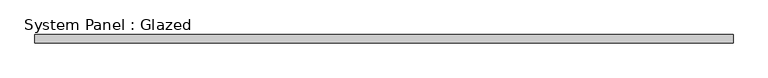
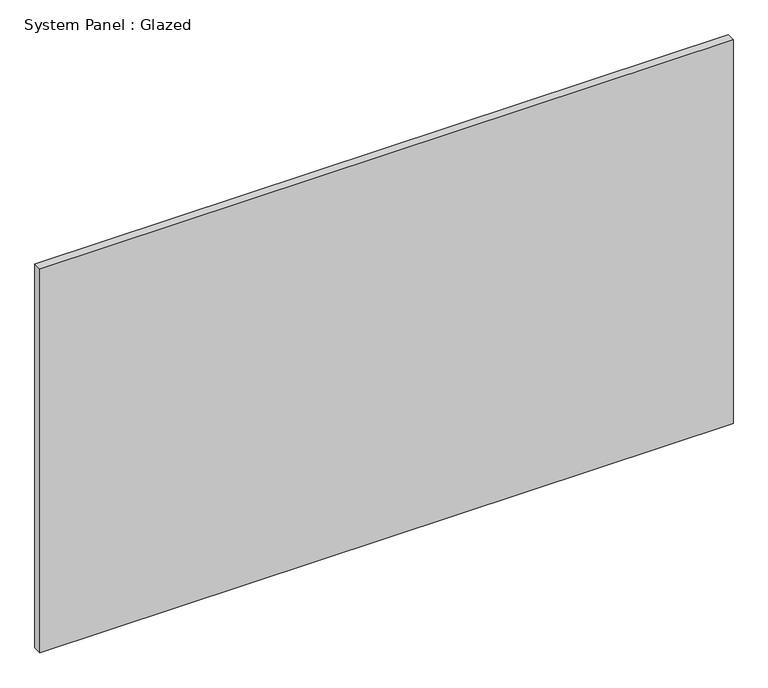
"""IFC4 building model written with IfcOpenShell, lengths in millimetres: plate geometry, System Panel : Glazed."""

from ifc_helpers import new_model, si_unit, origin, origin_with_axes, place, context, project, spatial, polyline, outline, extrude, source, transform, mapped, element, save


def system_panel_glazed_4fcd3a06(model_context):
    return source(origin(), model_context, "Body", "SweptSolid", [
        extrude(outline(polyline([(1041.4, 19.05), (-1041.4, 19.05), (-1041.4, 44.45), (1041.4, 44.45), (1041.4, 19.05)])), origin_with_axes(), (0.0, 0.0, 1.0), 1219.2),
    ])


if __name__ == "__main__":
    model = new_model("IFC4")
    model_context = context("Model", 3, world=origin())
    ifc_project = project(units=[si_unit("LENGTHUNIT", "METRE", prefix="MILLI")], contexts=[model_context])
    site = spatial("IfcSite", under=ifc_project)
    building = spatial("IfcBuilding", under=site)
    placement = place(None, origin())
    system_panel_glazed_shape = system_panel_glazed_4fcd3a06(model_context)
    element("IfcPlate", 1, ObjectType="System Panel : Glazed", at=placement, inside=building, context=model_context, shape_type="MappedRepresentation", body=[
        mapped(system_panel_glazed_shape, transform((0.0, 0.0, 0.0), x_axis=(1.0, 0.0, 0.0), y_axis=(0.0, 1.0, 0.0), z_axis=(0.0, 0.0, 1.0))),
    ])
    save(model, "model.ifc")

# Revit data of these elements
# Type "System Panel : Glazed"
#   Construction Type Id = "GSP4R"
#   Analytic Construction = "1/8 in Pilkington single glazing"
#   Visual Light Transmittance = 0.9
#   Solar Heat Gain Coefficient = 0.86
#   Heat Transfer Coefficient (U) = 1.18115 BTU/(h·ft²·°F)
# Element 1 (IfcPlate, "System Panel : Glazed")
#   Materials on its faces: "Glass"
# Materials
#   "Glass": class "Glass", colour RGB 0 128 192, transparency 0.75, Description = "Soda Lime Glass", Cost = 0
